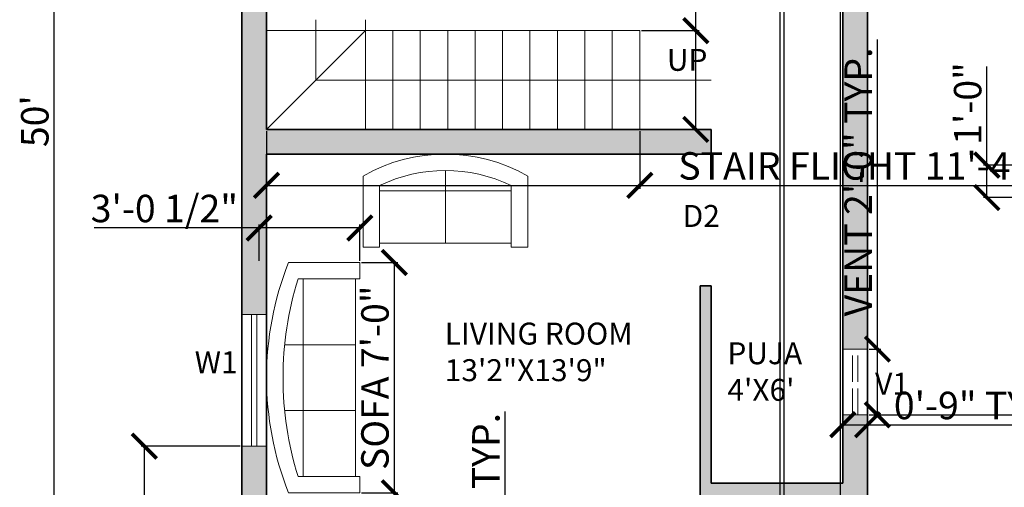
# Model space of a CAD drawing. Units: inches. Extents: x 2570 to 3313, y 1387 to 2106.
# Tile 2 of 5: x 2579 to 2938, y 1607 to 1777. Entities that reach past the tile are written whole.
import ezdxf

# ---------------------------------------------------------------- set-up
doc = ezdxf.new("R2010")
doc.units = ezdxf.units.IN
doc.linetypes.add('ACAD_ISO02W100', pattern=[15, 12, -3])
for name, color, linetype, lineweight in [('A-ANNO-DIMS', 7, 'Continuous', 18), ('A-ANNO-SYMB', 13, 'Continuous', 13), ('furniture', 11, 'Continuous', 18), ('STAIRS', 13, 'Continuous', 18), ('VENTILATORS', 143, 'ACAD_ISO02W100', 18), ('WALLS', 20, 'Continuous', 35), ('WINDOWS', 15, 'Continuous', 18)]:
    doc.layers.add(name, color=color, linetype=linetype, lineweight=lineweight)
for name, color, linetype, lineweight, true_color in [('A-ANNO-TEXT', 143, 'Continuous', 18, 0x7aafdf), ('A-AREA-IDEN', 143, 'Continuous', 18, 0x7aafdf), ('A-WALL-PATT', 30, 'Continuous', 13, 0xf26722)]:
    doc.layers.add(name, color=color, linetype=linetype, lineweight=lineweight, true_color=true_color)
doc.styles.get("Standard").update_dxf_attribs({"font": 'arial.ttf'})
doc.dimstyles.new('ISO-25', dxfattribs={"dimtxt": 10, "dimasz": 9, "dimexe": 1.25, "dimexo": 0.625, "dimtad": 1, "dimdec": 0, "dimlunit": 3, "dimtxsty": 'Standard', "dimblk": 'ARCHTICK', "dimcen": 2.5, "dimadec": 0, "dimazin": 0, "dimtfac": 1, "dimtdec": 0, "dimtmove": 0, "dimatfit": 3, "dimfxl": 1, "dimarcsym": 0})

# ---------------------------------------------------------------- blocks, each defined once
blk = doc.blocks.new('Sofa - Roundback Loveseat 5 ft.')
for p, q in [((0, -32.44198), (0, -5.99998)), ((-24, -33.99998), (-24, -11.46958)), ((-23.9998, -13.38178), (23.99986, -13.38178)), ((24.00004, -33.99998), (24.00004, -11.46958)), ((-24, -32.44198), (24.00004, -32.44198))]:
    blk.add_line(p, q)
for points in [[(-24, -33.99998), (-30, -33.99998), (-30, -7.99998)], [(30.00004, -7.99998), (30.00004, -33.99998), (24.00004, -33.99998)]]:
    blk.add_lwpolyline(points)
for centre, radius, start, end in [((0, -60.24998), 60.24998, 60.13715, 119.8628), ((0, -61.38438), 55.38444, 64.32083, 115.6792)]:
    blk.add_arc(centre, radius, start, end)
blk = doc.blocks.new('Sofa - Roundback 7 ft.')
for p, q in [((-12.00002, -32.4421), (-12.00003, -6.5971)), ((11.99997, -32.4421), (11.99998, -6.5971)), ((-36.000027, -34), (-36.000027, -11.4696)), ((-35.999844, -13.3819), (35.9998, -13.3819)), ((35.99998, -34), (35.99998, -11.4696)), ((-36.000027, -32.4421), (35.99998, -32.4421))]:
    blk.add_line(p, q)
for points in [[(-36.000027, -34), (-42.000027, -34), (-42.000027, -8)], [(41.99998, -8), (41.99998, -34), (35.99998, -34)]]:
    blk.add_lwpolyline(points)
for centre, radius, start, end in [((0, -114.25), 114.25, 68.43141, 111.5686), ((-0.00001, -127.1968), 121.1968, 72.72033, 107.2797)]:
    blk.add_arc(centre, radius, start, end)
blk = doc.blocks.new('_ArchTick')
at = {"color": 0, "linetype": 'ByBlock', "const_width": 0.15}
blk.add_lwpolyline([(-0.5, -0.5), (0.5, 0.5)], dxfattribs=at)
blk = doc.blocks.new('*D20')
at = {"layer": 'A-ANNO-DIMS', "color": 0, "lineweight": -2, "transparency": 16777216}
for p, q in [((2659.53, 2040.49), (2590.49, 2040.49)), ((2591.74, 1440.49), (2591.74, 2040.49)), ((2659.53, 1440.49), (2590.49, 1440.49))]:
    blk.add_line(p, q, dxfattribs=at)
at = {"layer": 'Defpoints', "color": 0, "transparency": 16777216}
for p in [(2591.74, 2040.49), (2660.15, 2040.49), (2660.15, 1440.49)]:
    blk.add_point(p, dxfattribs=at)
at = {"layer": 'A-ANNO-DIMS', "color": 0, "lineweight": -2, "transparency": 16777216, "xscale": 9, "yscale": 9, "zscale": 9}
for p, rotation in [((2591.74, 2040.49), 90), ((2591.74, 1440.49), 270)]:
    blk.add_blockref('_ArchTick', p, dxfattribs=dict(at, rotation=rotation))
at = {"layer": 'A-ANNO-DIMS', "color": 0, "transparency": 16777216, "insert": (2586.01, 1740.49), "char_height": 10, "attachment_point": 5, "rotation": 90}
blk.add_mtext("50'", dxfattribs=at)
blk = doc.blocks.new('WIN-48IN')
for p, q in [((-48, 0), (-48, -9)), ((0, 0), (0, -9)), ((0, -3.5), (-48, -3.5)), ((0, -5.5), (-48, -5.5))]:
    blk.add_line(p, q)
blk = doc.blocks.new('VENT-V1-24IN')
for p, q in [((0, 0), (9, 0)), ((0, -24), (9, -24))]:
    blk.add_line(p, q)
at = {"ltscale": 0.8}
for p, q in [((3.5, -24), (3.5, 0)), ((5.5, -24), (5.5, 0))]:
    blk.add_line(p, q, dxfattribs=at)
blk = doc.blocks.new('STAIR-FLIGHT-36IN-WINDER')
for p, q in [((136, 36), (0, 36)), ((36, 36), (0, 0)), ((36, 0), (36, 36)), ((46, 0), (46, 36)), ((56, 0), (56, 36)), ((66, 0), (66, 36)), ((76, 0), (76, 36)), ((86, 0), (86, 36)), ((96, 0), (96, 36)), ((106, 0), (106, 36)), ((116, 0), (116, 36)), ((126, 0), (126, 36)), ((136, 0), (136, 36))]:
    blk.add_line(p, q)
blk = doc.blocks.new('*D38')
at = {"layer": 'A-ANNO-DIMS', "color": 0, "lineweight": -2, "transparency": 16777216}
for p, q in [((2756.1, 1563.49), (2756.1, 1634.69)), ((2749.53, 1563.49), (2757.35, 1563.49)), ((2756.1, 1554.49), (2756.1, 1563.49)), ((2749.53, 1554.49), (2757.35, 1554.49))]:
    blk.add_line(p, q, dxfattribs=at)
at = {"layer": 'Defpoints', "color": 0, "transparency": 16777216}
for p in [(2748.9, 1563.49), (2756.1, 1563.49), (2748.9, 1554.49)]:
    blk.add_point(p, dxfattribs=at)
at = {"layer": 'A-ANNO-DIMS', "color": 0, "lineweight": -2, "transparency": 16777216, "xscale": 9, "yscale": 9, "zscale": 9}
for p, rotation in [((2756.1, 1563.49), 90), ((2756.1, 1554.49), 270)]:
    blk.add_blockref('_ArchTick', p, dxfattribs=dict(at, rotation=rotation))
at = {"layer": 'A-ANNO-DIMS', "color": 0, "transparency": 16777216, "insert": (2750.37, 1603.59), "char_height": 10, "attachment_point": 5, "rotation": 90}
blk.add_mtext('0\'-9" TYP.', dxfattribs=at)
blk = doc.blocks.new('*D43')
at = {"layer": 'A-ANNO-DIMS', "color": 0, "lineweight": -2, "transparency": 16777216}
for p, q in [((2891.75, 1657.4), (2891.75, 1770.26)), ((2888.78, 1657.4), (2893, 1657.4)), ((2891.75, 1633.4), (2891.75, 1657.4)), ((2888.78, 1633.4), (2893, 1633.4))]:
    blk.add_line(p, q, dxfattribs=at)
at = {"layer": 'Defpoints', "color": 0, "transparency": 16777216}
for p in [(2888.15, 1657.4), (2891.75, 1657.4), (2888.15, 1633.4)]:
    blk.add_point(p, dxfattribs=at)
at = {"layer": 'A-ANNO-DIMS', "color": 0, "lineweight": -2, "transparency": 16777216, "xscale": 9, "yscale": 9, "zscale": 9}
for p, rotation in [((2891.75, 1657.4), 90), ((2891.75, 1633.4), 270)]:
    blk.add_blockref('_ArchTick', p, dxfattribs=dict(at, rotation=rotation))
at = {"layer": 'A-ANNO-DIMS', "color": 0, "transparency": 16777216, "insert": (2886.02, 1718.33), "char_height": 10, "attachment_point": 5, "rotation": 90}
blk.add_mtext('VENT 2\'-0" TYP.', dxfattribs=at)
blk = doc.blocks.new('*D44')
at = {"layer": 'A-ANNO-DIMS', "color": 0, "lineweight": -2, "transparency": 16777216}
for p, q in [((2879.15, 1632.78), (2879.15, 1628.55)), ((2888.15, 1632.78), (2888.15, 1628.55)), ((2879.15, 1629.8), (2888.15, 1629.8)), ((2888.15, 1629.8), (2959.36, 1629.8))]:
    blk.add_line(p, q, dxfattribs=at)
at = {"layer": 'Defpoints', "color": 0, "transparency": 16777216}
for p in [(2879.15, 1633.4), (2888.15, 1633.4), (2888.15, 1629.8)]:
    blk.add_point(p, dxfattribs=at)
at = {"layer": 'A-ANNO-DIMS', "color": 0, "lineweight": -2, "transparency": 16777216, "xscale": 9, "yscale": 9, "zscale": 9, "rotation": 180}
blk.add_blockref('_ArchTick', (2879.15, 1629.8), dxfattribs=at)
at = {"layer": 'A-ANNO-DIMS', "color": 0, "lineweight": -2, "transparency": 16777216, "xscale": 9, "yscale": 9, "zscale": 9}
blk.add_blockref('_ArchTick', (2888.15, 1629.8), dxfattribs=at)
at = {"layer": 'A-ANNO-DIMS', "color": 0, "transparency": 16777216, "insert": (2928.26, 1635.53), "char_height": 10, "attachment_point": 5}
blk.add_mtext('0\'-9" TYP.', dxfattribs=at)
blk = doc.blocks.new('*D50')
at = {"layer": 'A-ANNO-DIMS', "color": 0, "lineweight": -2, "transparency": 16777216}
for p, q in [((2955.16, 1631.69), (2955.16, 1702.89)), ((2966.54, 1631.69), (2953.91, 1631.69)), ((2955.16, 1571.69), (2955.16, 1631.69)), ((2966.54, 1571.69), (2953.91, 1571.69))]:
    blk.add_line(p, q, dxfattribs=at)
at = {"layer": 'Defpoints', "color": 0, "transparency": 16777216}
for p in [(2955.16, 1631.69), (2967.16, 1631.69), (2967.16, 1571.69)]:
    blk.add_point(p, dxfattribs=at)
at = {"layer": 'A-ANNO-DIMS', "color": 0, "lineweight": -2, "transparency": 16777216, "xscale": 9, "yscale": 9, "zscale": 9}
for p, rotation in [((2955.16, 1631.69), 90), ((2955.16, 1571.69), 270)]:
    blk.add_blockref('_ArchTick', p, dxfattribs=dict(at, rotation=rotation))
at = {"layer": 'A-ANNO-DIMS', "color": 0, "transparency": 16777216, "insert": (2949.43, 1671.79), "char_height": 10, "attachment_point": 5, "rotation": 90}
blk.add_mtext('5\'-0" TYP.', dxfattribs=at)
blk = doc.blocks.new('*D53')
at = {"layer": 'A-ANNO-DIMS', "color": 0, "lineweight": -2, "transparency": 16777216}
for p, q in [((2669.15, 1736.86), (2669.15, 1715.84)), ((2805.15, 1736.86), (2805.15, 1715.84)), ((2669.15, 1717.09), (2805.15, 1717.09)), ((2805.15, 1717.09), (2982.66, 1717.09))]:
    blk.add_line(p, q, dxfattribs=at)
at = {"layer": 'Defpoints', "color": 0, "transparency": 16777216}
for p in [(2669.15, 1737.49), (2805.15, 1737.49), (2805.15, 1717.09)]:
    blk.add_point(p, dxfattribs=at)
at = {"layer": 'A-ANNO-DIMS', "color": 0, "lineweight": -2, "transparency": 16777216, "xscale": 9, "yscale": 9, "zscale": 9, "rotation": 180}
blk.add_blockref('_ArchTick', (2669.15, 1717.09), dxfattribs=at)
at = {"layer": 'A-ANNO-DIMS', "color": 0, "lineweight": -2, "transparency": 16777216, "xscale": 9, "yscale": 9, "zscale": 9}
blk.add_blockref('_ArchTick', (2805.15, 1717.09), dxfattribs=at)
at = {"layer": 'A-ANNO-DIMS', "color": 0, "transparency": 16777216, "insert": (2898.41, 1722.88), "char_height": 10, "attachment_point": 5}
blk.add_mtext('STAIR FLIGHT 11\'-4" TYP.', dxfattribs=at)
blk = doc.blocks.new('*D54')
at = {"layer": 'A-ANNO-DIMS', "color": 0, "lineweight": -2, "transparency": 16777216}
for p, q in [((2825.55, 1773.49), (2825.55, 1844.69)), ((2805.78, 1773.49), (2826.8, 1773.49)), ((2825.55, 1737.49), (2825.55, 1773.49)), ((2805.78, 1737.49), (2826.8, 1737.49))]:
    blk.add_line(p, q, dxfattribs=at)
at = {"layer": 'Defpoints', "color": 0, "transparency": 16777216}
for p in [(2805.15, 1773.49), (2825.55, 1773.49), (2805.15, 1737.49)]:
    blk.add_point(p, dxfattribs=at)
at = {"layer": 'A-ANNO-DIMS', "color": 0, "lineweight": -2, "transparency": 16777216, "xscale": 9, "yscale": 9, "zscale": 9}
for p, rotation in [((2825.55, 1773.49), 90), ((2825.55, 1737.49), 270)]:
    blk.add_blockref('_ArchTick', p, dxfattribs=dict(at, rotation=rotation))
at = {"layer": 'A-ANNO-DIMS', "color": 0, "transparency": 16777216, "insert": (2819.82, 1813.59), "char_height": 10, "attachment_point": 5, "rotation": 90}
blk.add_mtext('3\'-0" TYP.', dxfattribs=at)
blk = doc.blocks.new('*D59')
at = {"layer": 'A-ANNO-DIMS', "color": 0, "lineweight": -2, "transparency": 16777216}
for p, q in [((2703.78, 1688.95), (2717, 1688.95)), ((2715.75, 1604.95), (2715.75, 1688.95)), ((2703.78, 1604.95), (2717, 1604.95))]:
    blk.add_line(p, q, dxfattribs=at)
at = {"layer": 'Defpoints', "color": 0, "transparency": 16777216}
for p in [(2703.15, 1688.95), (2715.75, 1688.95), (2703.15, 1604.95)]:
    blk.add_point(p, dxfattribs=at)
at = {"layer": 'A-ANNO-DIMS', "color": 0, "lineweight": -2, "transparency": 16777216, "xscale": 9, "yscale": 9, "zscale": 9}
for p, rotation in [((2715.75, 1688.95), 90), ((2715.75, 1604.95), 270)]:
    blk.add_blockref('_ArchTick', p, dxfattribs=dict(at, rotation=rotation))
at = {"layer": 'A-ANNO-DIMS', "color": 0, "transparency": 16777216, "insert": (2709.95, 1646.95), "char_height": 10, "attachment_point": 5, "rotation": 90}
blk.add_mtext('SOFA 7\'-0"', dxfattribs=at)
blk = doc.blocks.new('*D60')
at = {"layer": 'A-ANNO-DIMS', "color": 0, "lineweight": -2, "transparency": 16777216}
for p, q in [((2666.48, 1701.55), (2606.36, 1701.55)), ((2666.48, 1689.58), (2666.48, 1702.8)), ((2703.15, 1701.55), (2666.48, 1701.55)), ((2703.15, 1689.58), (2703.15, 1702.8))]:
    blk.add_line(p, q, dxfattribs=at)
at = {"layer": 'Defpoints', "color": 0, "transparency": 16777216}
for p in [(2666.48, 1701.55), (2666.48, 1688.95), (2703.15, 1688.95)]:
    blk.add_point(p, dxfattribs=at)
at = {"layer": 'A-ANNO-DIMS', "color": 0, "lineweight": -2, "transparency": 16777216, "xscale": 9, "yscale": 9, "zscale": 9}
for p, rotation in [((2666.48, 1701.55), 180.0000221690003), ((2703.15, 1701.55), 2.21690002356e-05)]:
    blk.add_blockref('_ArchTick', p, dxfattribs=dict(at, rotation=rotation))
at = {"layer": 'A-ANNO-DIMS', "color": 0, "transparency": 16777216, "insert": (2631.92, 1707.35), "char_height": 10, "attachment_point": 5, "rotation": 0}
blk.add_mtext('3\'-0 1/2"', dxfattribs=at)
blk = doc.blocks.new('*D68')
at = {"layer": 'A-ANNO-DIMS', "color": 0, "lineweight": -2, "transparency": 16777216}
for p, q in [((2659.53, 1621.99), (2623.4, 1621.99)), ((2624.65, 1440.49), (2624.65, 1621.99)), ((2659.53, 1440.49), (2623.4, 1440.49))]:
    blk.add_line(p, q, dxfattribs=at)
at = {"layer": 'Defpoints', "color": 0, "transparency": 16777216}
for p in [(2624.65, 1621.99), (2660.15, 1621.99), (2660.15, 1440.49)]:
    blk.add_point(p, dxfattribs=at)
at = {"layer": 'A-ANNO-DIMS', "color": 0, "lineweight": -2, "transparency": 16777216, "xscale": 9, "yscale": 9, "zscale": 9}
for p, rotation in [((2624.65, 1621.99), 90), ((2624.65, 1440.49), 270)]:
    blk.add_blockref('_ArchTick', p, dxfattribs=dict(at, rotation=rotation))
at = {"layer": 'A-ANNO-DIMS', "color": 0, "transparency": 16777216, "insert": (2618.86, 1531.24), "char_height": 10, "attachment_point": 5, "rotation": 90}
blk.add_mtext('15\'-1 1/2"', dxfattribs=at)
blk = doc.blocks.new('*D76')
at = {"layer": 'A-ANNO-DIMS', "color": 0, "lineweight": -2, "transparency": 16777216}
for p, q in [((2888.78, 1633.4), (3222.91, 1633.4)), ((3221.66, 1440.49), (3221.66, 1633.4)), ((2888.78, 1440.49), (3222.91, 1440.49))]:
    blk.add_line(p, q, dxfattribs=at)
at = {"layer": 'Defpoints', "color": 0, "transparency": 16777216}
for p in [(2888.15, 1633.4), (3221.66, 1633.4), (2888.15, 1440.49)]:
    blk.add_point(p, dxfattribs=at)
at = {"layer": 'A-ANNO-DIMS', "color": 0, "lineweight": -2, "transparency": 16777216, "xscale": 9, "yscale": 9, "zscale": 9}
for p, rotation in [((3221.66, 1633.4), 90), ((3221.66, 1440.49), 270)]:
    blk.add_blockref('_ArchTick', p, dxfattribs=dict(at, rotation=rotation))
at = {"layer": 'A-ANNO-DIMS', "color": 0, "transparency": 16777216, "insert": (3215.93, 1536.94), "char_height": 10, "attachment_point": 5, "rotation": 90}
blk.add_mtext('16\'-1"', dxfattribs=at)
blk = doc.blocks.new('*D77')
at = {"layer": 'A-ANNO-DIMS', "color": 0, "lineweight": -2, "transparency": 16777216}
for p, q in [((2931.66, 1724.49), (2931.66, 1760.38)), ((2966.54, 1724.49), (2930.41, 1724.49)), ((2931.66, 1712.62), (2931.66, 1724.49)), ((2966.54, 1712.62), (2930.41, 1712.62))]:
    blk.add_line(p, q, dxfattribs=at)
at = {"layer": 'Defpoints', "color": 0, "transparency": 16777216}
for p in [(2931.66, 1724.49), (2967.16, 1724.49), (2967.16, 1712.62)]:
    blk.add_point(p, dxfattribs=at)
at = {"layer": 'A-ANNO-DIMS', "color": 0, "lineweight": -2, "transparency": 16777216, "xscale": 9, "yscale": 9, "zscale": 9}
for p, rotation in [((2931.66, 1724.49), 90), ((2931.66, 1712.62), 270)]:
    blk.add_blockref('_ArchTick', p, dxfattribs=dict(at, rotation=rotation))
at = {"layer": 'A-ANNO-DIMS', "color": 0, "transparency": 16777216, "insert": (2925.93, 1746.93), "char_height": 10, "attachment_point": 5, "rotation": 90}
blk.add_mtext('1\'-0"', dxfattribs=at)
blk = doc.blocks.new('*D81')
at = {"layer": 'A-ANNO-DIMS', "color": 0, "lineweight": -2, "transparency": 16777216}
for p, q in [((2856.15, 1873.66), (2856.15, 1403.74)), ((2878.15, 1873.66), (2878.15, 1403.74)), ((2856.15, 1404.99), (2878.15, 1404.99)), ((2878.15, 1404.99), (2921.82, 1404.99))]:
    blk.add_line(p, q, dxfattribs=at)
at = {"layer": 'Defpoints', "color": 0, "transparency": 16777216}
for p in [(2856.15, 1874.28), (2878.15, 1874.28), (2878.15, 1404.99)]:
    blk.add_point(p, dxfattribs=at)
at = {"layer": 'A-ANNO-DIMS', "color": 0, "lineweight": -2, "transparency": 16777216, "xscale": 9, "yscale": 9, "zscale": 9, "rotation": 180}
blk.add_blockref('_ArchTick', (2856.15, 1404.99), dxfattribs=at)
at = {"layer": 'A-ANNO-DIMS', "color": 0, "lineweight": -2, "transparency": 16777216, "xscale": 9, "yscale": 9, "zscale": 9}
blk.add_blockref('_ArchTick', (2878.15, 1404.99), dxfattribs=at)
at = {"layer": 'A-ANNO-DIMS', "color": 0, "transparency": 16777216, "insert": (2904.48, 1410.72), "char_height": 10, "attachment_point": 5}
blk.add_mtext('1\'-10"', dxfattribs=at)
blk = doc.blocks.new('*D83')
at = {"layer": 'A-ANNO-DIMS', "color": 0, "lineweight": -2, "transparency": 16777216}
for p, q in [((2857.69, 1934.86), (2857.69, 1403.74)), ((2878.15, 1934.86), (2878.15, 1403.74)), ((2857.69, 1404.99), (2878.15, 1404.99)), ((2878.15, 1404.99), (2937.35, 1404.99))]:
    blk.add_line(p, q, dxfattribs=at)
at = {"layer": 'Defpoints', "color": 0, "transparency": 16777216}
for p in [(2857.69, 1935.48), (2878.15, 1935.48), (2878.15, 1404.99)]:
    blk.add_point(p, dxfattribs=at)
at = {"layer": 'A-ANNO-DIMS', "color": 0, "lineweight": -2, "transparency": 16777216, "xscale": 9, "yscale": 9, "zscale": 9, "rotation": 180}
blk.add_blockref('_ArchTick', (2857.69, 1404.99), dxfattribs=at)
at = {"layer": 'A-ANNO-DIMS', "color": 0, "lineweight": -2, "transparency": 16777216, "xscale": 9, "yscale": 9, "zscale": 9}
blk.add_blockref('_ArchTick', (2878.15, 1404.99), dxfattribs=at)
at = {"layer": 'A-ANNO-DIMS', "color": 0, "transparency": 16777216, "insert": (2912.25, 1410.78), "char_height": 10, "attachment_point": 5}
blk.add_mtext('1\'-8 1/2"', dxfattribs=at)

msp = doc.modelspace()

# ---------------------------------------------------------------- hatches: boundary and pattern name
at = {"layer": 'A-WALL-PATT'}
h = msp.add_hatch(color=256, dxfattribs=at)
h.dxf.hatch_style = 1
h.paths.add_polyline_path([(2888.15, 1871.99), (2879.15, 1871.99), (2879.15, 1817.49), (2851.15, 1817.49), (2851.15, 1813.49), (2879.15, 1813.49), (2879.15, 1657.4), (2888.15, 1657.4)])
h.paths.add_polyline_path([(2831.15, 1737.49), (2669.15, 1737.49), (2669.15, 1813.49), (2745.15, 1813.49), (2745.15, 1849.49), (2741.15, 1849.49), (2741.15, 1817.49), (2669.15, 1817.49), (2669.15, 1838.62), (2660.15, 1838.62), (2660.15, 1669.99), (2669.15, 1669.99), (2669.15, 1728.49), (2831.15, 1728.49)])
h.paths.add_polyline_path([(2669.15, 1621.99), (2660.15, 1621.99), (2660.15, 1440.49), (2802.65, 1440.49), (2802.65, 1449.49), (2669.15, 1449.49), (2669.15, 1554.49), (2700.9, 1554.49), (2700.9, 1563.49), (2669.15, 1563.49)])
h.paths.add_polyline_path([(2780.65, 1563.49), (2748.9, 1563.49), (2748.9, 1554.49), (2780.65, 1554.49)], flags=17)
h.paths.add_polyline_path([(2836.15, 1599.49), (2879.15, 1599.49), (2879.15, 1449.49), (2874.65, 1449.49), (2874.65, 1440.49), (2888.15, 1440.49), (2888.15, 1633.4), (2879.15, 1633.4), (2879.15, 1608.49), (2831.15, 1608.49), (2831.15, 1680.49), (2827.15, 1680.49), (2827.15, 1563.49), (2822.65, 1563.49), (2822.65, 1554.49), (2836.15, 1554.49)])
h.paths.add_polyline_path([(2793.15, 1962.49), (2821.15, 1962.49), (2821.15, 1971.49), (2793.15, 1971.49), (2793.15, 2031.49), (2818.15, 2031.49), (2818.15, 2040.49), (2747.15, 2040.49), (2747.15, 2031.49), (2789.15, 2031.49), (2789.15, 1887.49), (2785.15, 1887.49), (2785.15, 1879.49), (2789.15, 1879.49), (2789.15, 1817.49), (2789.15, 1813.49), (2793.15, 1813.49), (2821.15, 1813.49), (2821.15, 1817.49), (2793.15, 1817.49)])
h.paths.add_polyline_path([(2749.15, 1887.49), (2669.15, 1887.49), (2669.15, 2031.49), (2711.15, 2031.49), (2711.15, 2040.49), (2660.15, 2040.49), (2660.15, 1862.62), (2669.15, 1862.62), (2669.15, 1883.49), (2741.15, 1883.49), (2741.15, 1879.49), (2749.15, 1879.49)])
h.paths.add_polyline_path([(2888.15, 2040.49), (2854.15, 2040.49), (2854.15, 2031.49), (2879.15, 2031.49), (2879.15, 1971.49), (2877.15, 1971.49), (2877.15, 1962.49), (2879.15, 1962.49), (2879.15, 1907.99), (2888.15, 1907.99)])
h.paths.add_polyline_path([(2967.16, 2031.49), (3011.16, 2031.49), (3011.16, 2004.49), (3015.16, 2004.49), (3015.16, 2031.49), (3039.26, 2031.49), (3039.26, 2040.49), (2958.16, 2040.49), (2958.16, 1909.99), (2967.16, 1909.99), (2967.16, 1921.99), (2967.16, 1966.49)])
h.paths.add_polyline_path([(3186.16, 2040.49), (3063.26, 2040.49), (3063.26, 2031.49), (3087.16, 2031.49), (3087.16, 1970.49), (3015.16, 1970.49), (3015.16, 1974.49), (3011.16, 1974.49), (3011.16, 1966.49), (3177.16, 1966.49), (3177.16, 1817.49), (3172.66, 1817.49), (3172.66, 1813.49), (3177.16, 1813.49), (3177.16, 1721.56), (3186.16, 1721.56)])
h.paths.add_polyline_path([(3177.16, 2031.49), (3177.16, 1970.49), (3091.16, 1970.49), (3091.16, 2031.49)], flags=16)
h.paths.add_polyline_path([(2967.16, 1873.99), (2958.16, 1873.99), (2958.16, 1712.62), (2967.16, 1712.62), (2967.16, 1724.49), (3051.16, 1724.49), (3051.16, 1710.49), (3055.16, 1710.49), (3055.16, 1724.49), (3125.16, 1724.49), (3125.16, 1676.49), (3085.16, 1676.49), (3085.16, 1672.49), (3125.16, 1672.49), (3125.16, 1668.49), (3129.16, 1668.49), (3129.16, 1733.49), (2967.16, 1733.49), (2967.16, 1813.49), (3136.66, 1813.49), (3136.66, 1817.49), (2967.16, 1817.49)])
h.paths.add_polyline_path([(2967.16, 1672.49), (3055.16, 1672.49), (3055.16, 1680.49), (3051.16, 1680.49), (3051.16, 1676.49), (2967.16, 1676.49), (2967.16, 1688.62), (2958.16, 1688.62), (2958.16, 1618.49), (2967.16, 1618.49), (2967.16, 1631.69)])
h.paths.add_polyline_path([(3186.16, 1685.56), (3177.16, 1685.56), (3177.16, 1568.09), (3169.16, 1568.09), (3169.16, 1564.09), (3177.16, 1564.09), (3177.16, 1519.49), (3177.16, 1449.49), (3186.16, 1449.49)])
h.paths.add_polyline_path([(3129.16, 1564.09), (3129.16, 1632.49), (3125.16, 1632.49), (3125.16, 1528.49), (2967.16, 1528.49), (2967.16, 1582.49), (2958.16, 1582.49), (2958.16, 1449.49), (2967.16, 1449.49), (2967.16, 1519.49), (3129.16, 1519.49)])
h.paths.add_polyline_path([(3123.16, 1975.63), (3150.13, 1975.63), (3150.13, 1992.12), (3123.16, 1992.12)], flags=8)
h.paths.add_polyline_path([(3130.18, 1590.82), (3180.42, 1590.82), (3180.42, 1617.03), (3130.18, 1617.03)], flags=9)

# ---------------------------------------------------------------- linework, layer by layer
at = {"layer": 'A-ANNO-SYMB'}
for p, q in [((2687.15, 1773.49), (2687.15, 1777.49)), ((2687.15, 1755.49), (2687.15, 1773.49)), ((2831.15, 1755.49), (2687.15, 1755.49))]:
    msp.add_line(p, q, dxfattribs=at)
at = {"layer": 'STAIRS'}
msp.add_line((2705.15, 1773.49), (2705.15, 1777.49), dxfattribs=at)
at = {"layer": 'WALLS'}
for p, q in [((2660.15, 1440.49), (2660.15, 2040.49)), ((2888.15, 2040.49), (2888.15, 1440.49)), ((2669.15, 1737.49), (2669.15, 1813.49)), ((2879.15, 1813.49), (2879.15, 1608.49)), ((2831.15, 1737.49), (2669.15, 1737.49)), ((2831.15, 1737.49), (2831.15, 1728.49)), ((2831.15, 1728.49), (2669.15, 1728.49)), ((2669.15, 1563.49), (2669.15, 1728.49)), ((2827.15, 1563.49), (2827.15, 1680.49)), ((2831.15, 1680.49), (2827.15, 1680.49)), ((2831.15, 1608.49), (2831.15, 1680.49)), ((2879.15, 1608.49), (2831.15, 1608.49))]:
    msp.add_line(p, q, dxfattribs=at)

# ---------------------------------------------------------------- block references
at = {"layer": 'furniture'}
msp.add_blockref('Sofa - Roundback Loveseat 5 ft.', (2734.31, 1728.49), dxfattribs=at)
at = {"layer": 'furniture', "rotation": 90.00002216900027}
msp.add_blockref('Sofa - Roundback 7 ft.', (2669.15, 1646.95), dxfattribs=at)
at = {"layer": 'STAIRS'}
msp.add_blockref('STAIR-FLIGHT-36IN-WINDER', (2669.15, 1737.49), dxfattribs=at)
at = {"layer": 'VENTILATORS'}
msp.add_blockref('VENT-V1-24IN', (2879.15, 1657.4), dxfattribs=at)
at = {"layer": 'WINDOWS', "rotation": 90.00000000000003}
msp.add_blockref('WIN-48IN', (2660.15, 1669.99), dxfattribs=at)

# ---------------------------------------------------------------- texts
at = {"layer": 'A-ANNO-TEXT', "char_height": 8, "attachment_point": 1}
for s, width, insert in [('UP', 60.8198, (2815.02, 1766.84)), ('D2', 13.0839, (2820.78, 1709.92)), ('W1', 13.4987, (2642.97, 1656.58)), ('V1', 13.4987, (2890.9, 1648.75))]:
    msp.add_mtext_dynamic_manual_height_columns(s, width=width, gutter_width=12.5, heights=[0], dxfattribs=dict(at, insert=insert))
at = {"layer": 'A-AREA-IDEN', "char_height": 8, "attachment_point": 1}
for s, width, insert in [('LIVING ROOM\\P13\'2"X13\'9"', 174.4785, (2734.09, 1667.03)), ("PUJA\\P4'X6'", 60.8198, (2837.08, 1659.87))]:
    msp.add_mtext_dynamic_manual_height_columns(s, width=width, gutter_width=12.5, heights=[0], dxfattribs=dict(at, insert=insert))

# ---------------------------------------------------------------- dimensions: what is measured, and where the dimension line sits
at = {"layer": 'A-ANNO-DIMS'}
for base, p1, p2, angle, override, picture, middle in [((2591.74, 2040.49), (2660.15, 1440.49), (2660.15, 2040.49), 90, {"dimclrd": 0, "dimclre": 0, "dimclrt": 0}, '*D20', (2586.01, 1740.49)), ((2931.66, 1724.49), (2967.16, 1712.62), (2967.16, 1724.49), 90, {"dimdec": 1, "dimlfac": 1, "dimrnd": 0, "dimzin": 1, "dimdsep": 46, "dimlunit": 4, "dimfrac": 2}, '*D77', (2925.93, 1746.93)), ((2666.48, 1701.55), (2703.15, 1688.95), (2666.48, 1688.95), 180, {"dimdec": 1, "dimlfac": 1, "dimrnd": 0, "dimzin": 1, "dimdsep": 46, "dimlunit": 4, "dimfrac": 2}, '*D60', (2631.92, 1707.35)), ((3221.66, 1633.4), (2888.15, 1440.49), (2888.15, 1633.4), 90, {"dimdec": 1, "dimlfac": 1, "dimrnd": 0, "dimzin": 1, "dimdsep": 46, "dimlunit": 4, "dimfrac": 2}, '*D76', (3215.93, 1536.94)), ((2624.65, 1621.99), (2660.15, 1440.49), (2660.15, 1621.99), 90, {"dimdec": 1, "dimlfac": 1, "dimrnd": 0, "dimzin": 1, "dimdsep": 46, "dimlunit": 4, "dimfrac": 2}, '*D68', (2618.86, 1531.24))]:
    dim = msp.add_linear_dim(base=base, p1=p1, p2=p2, angle=angle, dimstyle='ISO-25', override=override, dxfattribs=at)
    dim.commit()
    dim.dimension.update_dxf_attribs({"geometry": picture, "text_midpoint": middle})
for p1, p2, picture, middle in [((2857.69, 1935.48), (2878.15, 1935.48), '*D83', (2912.25, 1410.78)), ((2856.15, 1874.28), (2878.15, 1874.28), '*D81', (2904.48, 1410.72))]:
    dim = msp.add_linear_dim(base=(2878.15, 1404.99), p1=p1, p2=p2, dimstyle='ISO-25', override={"dimdec": 1, "dimlfac": 1, "dimrnd": 0, "dimzin": 1, "dimdsep": 46, "dimlunit": 4, "dimfrac": 2}, dxfattribs=at)
    dim.commit()
    dim.dimension.update_dxf_attribs({"geometry": picture, "text_midpoint": middle})
for base, p1, p2, text, picture, middle in [((2825.55, 1773.49), (2805.15, 1737.49), (2805.15, 1773.49), '<> TYP.', '*D54', (2819.82, 1813.59)), ((2891.75, 1657.4), (2888.15, 1633.4), (2888.15, 1657.4), 'VENT <> TYP.', '*D43', (2886.02, 1718.33)), ((2955.16, 1631.69), (2967.16, 1571.69), (2967.16, 1631.69), '<> TYP.', '*D50', (2949.43, 1671.79)), ((2715.75, 1688.95), (2703.15, 1604.95), (2703.15, 1688.95), 'SOFA <>', '*D59', (2709.95, 1646.95)), ((2756.1, 1563.49), (2748.9, 1554.49), (2748.9, 1563.49), '<> TYP.', '*D38', (2750.37, 1603.59))]:
    dim = msp.add_linear_dim(base=base, p1=p1, p2=p2, angle=90, text=text, dimstyle='ISO-25', override={"dimdec": 1, "dimlfac": 1, "dimrnd": 0, "dimzin": 1, "dimdsep": 46, "dimlunit": 4, "dimfrac": 2}, dxfattribs=at)
    dim.commit()
    dim.dimension.update_dxf_attribs({"geometry": picture, "text_midpoint": middle})
for base, p1, p2, text, picture, middle in [((2805.15, 1717.09), (2669.15, 1737.49), (2805.15, 1737.49), 'STAIR FLIGHT <> TYP.', '*D53', (2898.41, 1722.88)), ((2888.15, 1629.8), (2879.15, 1633.4), (2888.15, 1633.4), '<> TYP.', '*D44', (2928.26, 1635.53))]:
    dim = msp.add_linear_dim(base=base, p1=p1, p2=p2, text=text, dimstyle='ISO-25', override={"dimdec": 1, "dimlfac": 1, "dimrnd": 0, "dimzin": 1, "dimdsep": 46, "dimlunit": 4, "dimfrac": 2}, dxfattribs=at)
    dim.commit()
    dim.dimension.update_dxf_attribs({"geometry": picture, "text_midpoint": middle})

doc.saveas('drawing.dxf')
